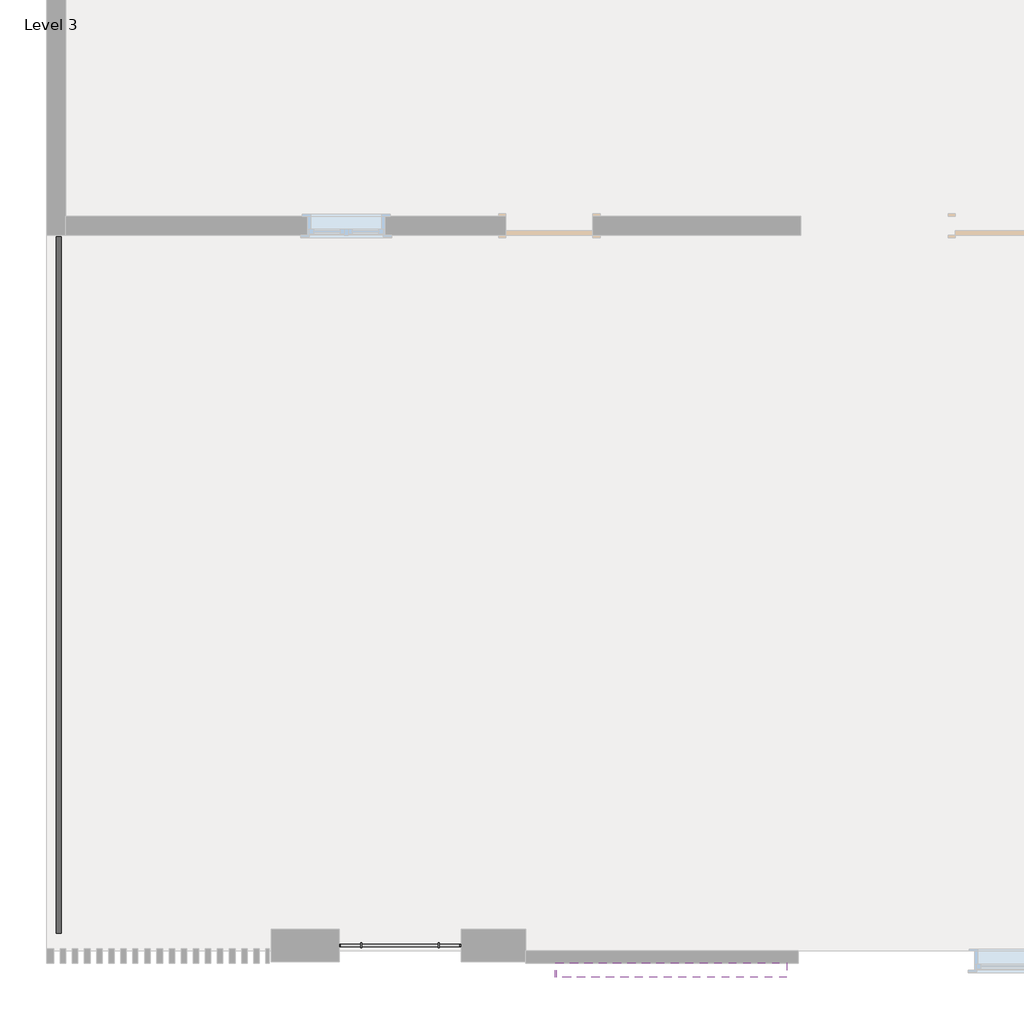
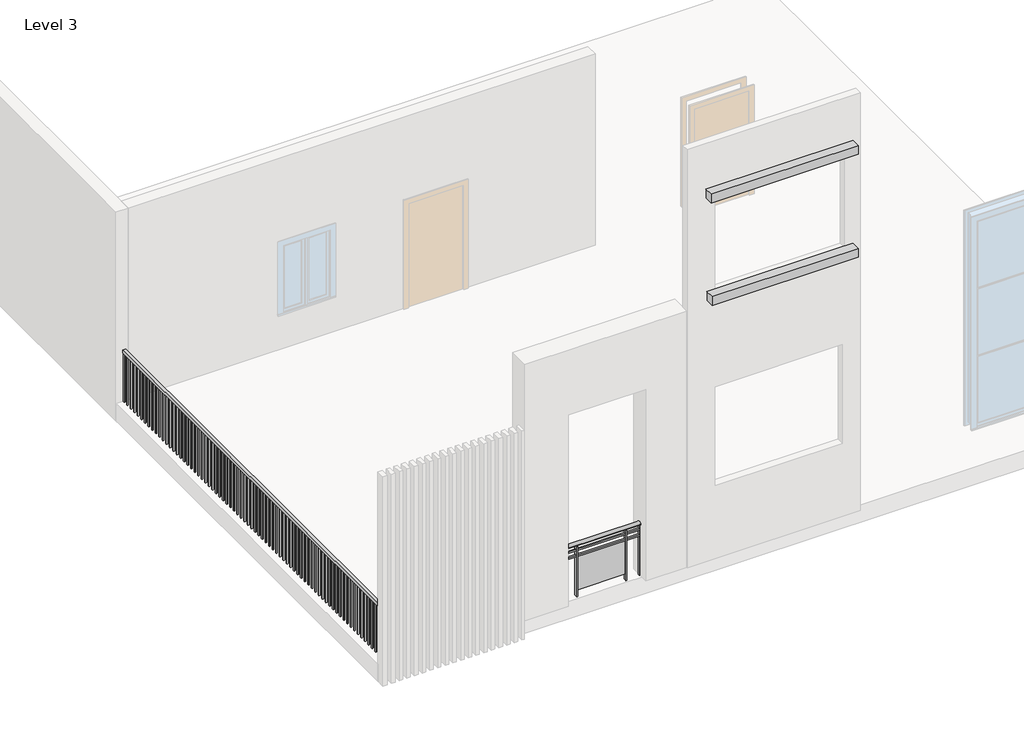
# One storey, part 2 of 2: 2 proxies, 2 railings.
"""IFC4 building model written with IfcOpenShell, lengths in millimetres."""

from ifc_helpers import new_model, si_unit, point, frame, origin, place, context, project, spatial, polyline, ellipse_curve, trimmed, outline, extrude, element, save
from ifc_brep_helpers import plane_surface, extruded_surface, advanced_brep

model = new_model("IFC4")

# Units and contexts
model_context = context("Model", 3, world=origin())
ifc_project = project(units=[si_unit("LENGTHUNIT", "METRE", prefix="MILLI")], contexts=[model_context])

# Site, building, storey
site = spatial("IfcSite", under=ifc_project)
building = spatial("IfcBuilding", under=site)
storey = spatial("IfcBuildingStorey", under=building, Name="Level 3", Elevation=7315.2)

# Proxies
placement = place(None, origin())
element("IfcBuildingElementProxy", 1, Name="Cornice", ObjectType="Cornice", at=placement, inside=storey, context=model_context, shape_type="SweptSolid", body=[
    extrude(outline(polyline([(-6506.8547188, -1061.9189974), (-6506.8547188, -909.5189974), (-4073.2084212, -909.5189974), (-4073.2084212, -1061.9189974), (-6506.8547188, -1061.9189974)])), frame((0.0, 0.0, 13989.7022407), z_axis=(0.0, 0.0, 1.0), x_axis=(1.0, 0.0, 0.0)), (0.0, 0.0, 1.0), 152.4),
])
element("IfcBuildingElementProxy", 2, Name="Cornice", ObjectType="Cornice", at=placement, inside=storey, context=model_context, shape_type="SweptSolid", body=[
    extrude(outline(polyline([(-6490.544029, -1061.9189974), (-6490.544029, -909.5189974), (-4073.2084212, -909.5189974), (-4073.2084212, -1061.9189974), (-6490.544029, -1061.9189974)])), frame((0.0, 0.0, 12192.0), z_axis=(0.0, 0.0, 1.0), x_axis=(1.0, 0.0, 0.0)), (0.0, 0.0, 1.0), 152.4),
])

# Railings
element("IfcRailing", 3, ObjectType="Glass Panel - Bottom Fill", at=placement, inside=storey, context=model_context, shape_type="SolidModel", body=[
    advanced_brep(
    [(-8777.0745124, -686.4386035, 8534.4), (-8777.0745124, -762.6386035, 8534.4), (-7495.2589248, -686.4386035, 8534.4), (-7495.2589248, -762.6386035, 8534.4)],
    [
        (0, 1, ellipse_curve(frame((-8777.0745124, -724.5386035, 8534.4), z_axis=(-1.0, 0.0, 0.0), x_axis=(0.0, -1.0, 0.0)), 38.1, 28.575)),
        (1, 0, ellipse_curve(frame((-8777.0745124, -724.5386035, 8534.4), z_axis=(-1.0, 0.0, 0.0), x_axis=(0.0, -1.0, 0.0)), 38.1, 28.575)),
        (2, 3, ellipse_curve(frame((-7495.2589248, -724.5386035, 8534.4), z_axis=(1.0, 0.0, 0.0), x_axis=(0.0, -1.0, 0.0)), 38.1, 28.575)),
        (3, 2, ellipse_curve(frame((-7495.2589248, -724.5386035, 8534.4), z_axis=(1.0, 0.0, 0.0), x_axis=(0.0, -1.0, 0.0)), 38.1, 28.575)),
        (0, 2),
        (3, 1),
    ],
    [
        plane_surface(frame((-8777.0745124, -724.5386035, 8534.4), z_axis=(-1.0, 0.0, 0.0), x_axis=(0.0, 1.0, 0.0))),
        plane_surface(frame((-7495.2589248, -724.5386035, 8534.4), z_axis=(1.0, 0.0, 0.0), x_axis=(0.0, 1.0, 0.0))),
        extruded_surface(trimmed(ellipse_curve(frame((-7495.2589248, -724.5386035, 8534.4), z_axis=(-1.0, 0.0, 0.0), x_axis=(0.0, -1.0, 0.0)), 38.1, 28.575), [point((-7495.2589248, -686.4386035, 8534.4))], [point((-7495.2589248, -762.6386035, 8534.4))], True, "CARTESIAN"), (-1281.8155876, 0.0, 0.0), 1281.8155876),
        extruded_surface(trimmed(ellipse_curve(frame((-7495.2589248, -724.5386035, 8534.4), z_axis=(-1.0, 0.0, 0.0), x_axis=(0.0, -1.0, 0.0)), 38.1, 28.575), [point((-7495.2589248, -762.6386035, 8534.4))], [point((-7495.2589248, -686.4386035, 8534.4))], True, "CARTESIAN"), (-1281.8155876, 0.0, 0.0), 1281.8155876),
    ],
    [
        (0, [[1, 2]]),
        (1, [[3, 4]]),
        (2, [[-1, 5, -4, 6]]),
        (3, [[-2, -6, -3, -5]]),
    ],
),
    extrude(outline(polyline([(-8777.0745124, -737.2386035), (-8777.0745124, -711.8386035), (-7495.2589248, -711.8386035), (-7495.2589248, -737.2386035), (-8777.0745124, -737.2386035)])), frame((0.0, 0.0, 8420.1), z_axis=(0.0, 0.0, 1.0), x_axis=(1.0, 0.0, 0.0)), (0.0, 0.0, 1.0), 25.4),
    extrude(outline(polyline([(-8777.0745124, -737.2386035), (-8777.0745124, -711.8386035), (-7495.2589248, -711.8386035), (-7495.2589248, -737.2386035), (-8777.0745124, -737.2386035)])), frame((0.0, 0.0, 8318.5), z_axis=(0.0, 0.0, 1.0), x_axis=(1.0, 0.0, 0.0)), (0.0, 0.0, 1.0), 25.4),
    extrude(outline(polyline([(-7736.1167186, -749.9386035), (-7736.1167186, -699.1386035), (-7723.4167186, -699.1386035), (-7723.4167186, -749.9386035), (-7736.1167186, -749.9386035)])), frame((0.0, 0.0, 7620.0), z_axis=(0.0, 0.0, 1.0), x_axis=(1.0, 0.0, 0.0)), (0.0, 0.0, 1.0), 885.6788223),
    extrude(outline(polyline([(-8542.5667186, -718.0034465), (-7729.7667186, -718.0034465), (-7729.7667186, -724.3534465), (-8542.5667186, -724.3534465), (-8542.5667186, -718.0034465)])), frame((0.0, 0.0, 7721.6), z_axis=(0.0, 0.0, 1.0), x_axis=(1.0, 0.0, 0.0)), (0.0, 0.0, 1.0), 596.9),
    extrude(outline(polyline([(-8548.9167186, -749.9386035), (-8548.9167186, -699.1386035), (-8536.2167186, -699.1386035), (-8536.2167186, -749.9386035), (-8548.9167186, -749.9386035)])), frame((0.0, 0.0, 7620.0), z_axis=(0.0, 0.0, 1.0), x_axis=(1.0, 0.0, 0.0)), (0.0, 0.0, 1.0), 885.6788223),
    extrude(outline(polyline([(-7507.9589248, -734.0636035), (-7507.9589248, -715.0136035), (-7488.9089248, -715.0136035), (-7488.9089248, -734.0636035), (-7507.9589248, -734.0636035)])), frame((0.0, 0.0, 7620.0), z_axis=(0.0, 0.0, 1.0), x_axis=(1.0, 0.0, 0.0)), (0.0, 0.0, 1.0), 885.6788223),
    extrude(outline(polyline([(-8783.4245124, -734.0636035), (-8783.4245124, -715.0136035), (-8764.3745124, -715.0136035), (-8764.3745124, -734.0636035), (-8783.4245124, -734.0636035)])), frame((0.0, 0.0, 7620.0), z_axis=(0.0, 0.0, 1.0), x_axis=(1.0, 0.0, 0.0)), (0.0, 0.0, 1.0), 885.6788223),
])
element("IfcRailing", 4, ObjectType="Handrail - Rectangular", at=placement, inside=storey, context=model_context, shape_type="SweptSolid", body=[
    extrude(outline(polyline([(-11748.8745124, 6720.6131791), (-11698.0745124, 6720.6131791), (-11698.0745124, -594.5868209), (-11748.8745124, -594.5868209), (-11748.8745124, 6720.6131791)])), frame((0.0, 0.0, 8483.6), z_axis=(0.0, 0.0, 1.0), x_axis=(1.0, 0.0, 0.0)), (0.0, 0.0, 1.0), 50.8),
    extrude(outline(polyline([(-11732.9995124, -483.4618209), (-11713.9495124, -483.4618209), (-11713.9495124, -502.5118209), (-11732.9995124, -502.5118209), (-11732.9995124, -483.4618209)])), frame((0.0, 0.0, 7620.0), z_axis=(0.0, 0.0, 1.0), x_axis=(1.0, 0.0, 0.0)), (0.0, 0.0, 1.0), 863.6),
    extrude(outline(polyline([(-11732.9995124, -381.8618209), (-11713.9495124, -381.8618209), (-11713.9495124, -400.9118209), (-11732.9995124, -400.9118209), (-11732.9995124, -381.8618209)])), frame((0.0, 0.0, 7620.0), z_axis=(0.0, 0.0, 1.0), x_axis=(1.0, 0.0, 0.0)), (0.0, 0.0, 1.0), 863.6),
    extrude(outline(polyline([(-11732.9995124, -280.2618209), (-11713.9495124, -280.2618209), (-11713.9495124, -299.3118209), (-11732.9995124, -299.3118209), (-11732.9995124, -280.2618209)])), frame((0.0, 0.0, 7620.0), z_axis=(0.0, 0.0, 1.0), x_axis=(1.0, 0.0, 0.0)), (0.0, 0.0, 1.0), 863.6),
    extrude(outline(polyline([(-11732.9995124, -178.6618209), (-11713.9495124, -178.6618209), (-11713.9495124, -197.7118209), (-11732.9995124, -197.7118209), (-11732.9995124, -178.6618209)])), frame((0.0, 0.0, 7620.0), z_axis=(0.0, 0.0, 1.0), x_axis=(1.0, 0.0, 0.0)), (0.0, 0.0, 1.0), 863.6),
    extrude(outline(polyline([(-11732.9995124, -77.0618209), (-11713.9495124, -77.0618209), (-11713.9495124, -96.1118209), (-11732.9995124, -96.1118209), (-11732.9995124, -77.0618209)])), frame((0.0, 0.0, 7620.0), z_axis=(0.0, 0.0, 1.0), x_axis=(1.0, 0.0, 0.0)), (0.0, 0.0, 1.0), 863.6),
    extrude(outline(polyline([(-11732.9995124, 24.5381791), (-11713.9495124, 24.5381791), (-11713.9495124, 5.4881791), (-11732.9995124, 5.4881791), (-11732.9995124, 24.5381791)])), frame((0.0, 0.0, 7620.0), z_axis=(0.0, 0.0, 1.0), x_axis=(1.0, 0.0, 0.0)), (0.0, 0.0, 1.0), 863.6),
    extrude(outline(polyline([(-11732.9995124, 126.1381791), (-11713.9495124, 126.1381791), (-11713.9495124, 107.0881791), (-11732.9995124, 107.0881791), (-11732.9995124, 126.1381791)])), frame((0.0, 0.0, 7620.0), z_axis=(0.0, 0.0, 1.0), x_axis=(1.0, 0.0, 0.0)), (0.0, 0.0, 1.0), 863.6),
    extrude(outline(polyline([(-11732.9995124, 227.7381791), (-11713.9495124, 227.7381791), (-11713.9495124, 208.6881791), (-11732.9995124, 208.6881791), (-11732.9995124, 227.7381791)])), frame((0.0, 0.0, 7620.0), z_axis=(0.0, 0.0, 1.0), x_axis=(1.0, 0.0, 0.0)), (0.0, 0.0, 1.0), 863.6),
    extrude(outline(polyline([(-11732.9995124, 329.3381791), (-11713.9495124, 329.3381791), (-11713.9495124, 310.2881791), (-11732.9995124, 310.2881791), (-11732.9995124, 329.3381791)])), frame((0.0, 0.0, 7620.0), z_axis=(0.0, 0.0, 1.0), x_axis=(1.0, 0.0, 0.0)), (0.0, 0.0, 1.0), 863.6),
    extrude(outline(polyline([(-11732.9995124, 430.9381791), (-11713.9495124, 430.9381791), (-11713.9495124, 411.8881791), (-11732.9995124, 411.8881791), (-11732.9995124, 430.9381791)])), frame((0.0, 0.0, 7620.0), z_axis=(0.0, 0.0, 1.0), x_axis=(1.0, 0.0, 0.0)), (0.0, 0.0, 1.0), 863.6),
    extrude(outline(polyline([(-11732.9995124, 532.5381791), (-11713.9495124, 532.5381791), (-11713.9495124, 513.4881791), (-11732.9995124, 513.4881791), (-11732.9995124, 532.5381791)])), frame((0.0, 0.0, 7620.0), z_axis=(0.0, 0.0, 1.0), x_axis=(1.0, 0.0, 0.0)), (0.0, 0.0, 1.0), 863.6),
    extrude(outline(polyline([(-11732.9995124, 634.1381791), (-11713.9495124, 634.1381791), (-11713.9495124, 615.0881791), (-11732.9995124, 615.0881791), (-11732.9995124, 634.1381791)])), frame((0.0, 0.0, 7620.0), z_axis=(0.0, 0.0, 1.0), x_axis=(1.0, 0.0, 0.0)), (0.0, 0.0, 1.0), 863.6),
    extrude(outline(polyline([(-11732.9995124, 735.7381791), (-11713.9495124, 735.7381791), (-11713.9495124, 716.6881791), (-11732.9995124, 716.6881791), (-11732.9995124, 735.7381791)])), frame((0.0, 0.0, 7620.0), z_axis=(0.0, 0.0, 1.0), x_axis=(1.0, 0.0, 0.0)), (0.0, 0.0, 1.0), 863.6),
    extrude(outline(polyline([(-11732.9995124, 837.3381791), (-11713.9495124, 837.3381791), (-11713.9495124, 818.2881791), (-11732.9995124, 818.2881791), (-11732.9995124, 837.3381791)])), frame((0.0, 0.0, 7620.0), z_axis=(0.0, 0.0, 1.0), x_axis=(1.0, 0.0, 0.0)), (0.0, 0.0, 1.0), 863.6),
    extrude(outline(polyline([(-11732.9995124, 938.9381791), (-11713.9495124, 938.9381791), (-11713.9495124, 919.8881791), (-11732.9995124, 919.8881791), (-11732.9995124, 938.9381791)])), frame((0.0, 0.0, 7620.0), z_axis=(0.0, 0.0, 1.0), x_axis=(1.0, 0.0, 0.0)), (0.0, 0.0, 1.0), 863.6),
    extrude(outline(polyline([(-11732.9995124, 1040.5381791), (-11713.9495124, 1040.5381791), (-11713.9495124, 1021.4881791), (-11732.9995124, 1021.4881791), (-11732.9995124, 1040.5381791)])), frame((0.0, 0.0, 7620.0), z_axis=(0.0, 0.0, 1.0), x_axis=(1.0, 0.0, 0.0)), (0.0, 0.0, 1.0), 863.6),
    extrude(outline(polyline([(-11732.9995124, 1142.1381791), (-11713.9495124, 1142.1381791), (-11713.9495124, 1123.0881791), (-11732.9995124, 1123.0881791), (-11732.9995124, 1142.1381791)])), frame((0.0, 0.0, 7620.0), z_axis=(0.0, 0.0, 1.0), x_axis=(1.0, 0.0, 0.0)), (0.0, 0.0, 1.0), 863.6),
    extrude(outline(polyline([(-11732.9995124, 1243.7381791), (-11713.9495124, 1243.7381791), (-11713.9495124, 1224.6881791), (-11732.9995124, 1224.6881791), (-11732.9995124, 1243.7381791)])), frame((0.0, 0.0, 7620.0), z_axis=(0.0, 0.0, 1.0), x_axis=(1.0, 0.0, 0.0)), (0.0, 0.0, 1.0), 863.6),
    extrude(outline(polyline([(-11732.9995124, 1345.3381791), (-11713.9495124, 1345.3381791), (-11713.9495124, 1326.2881791), (-11732.9995124, 1326.2881791), (-11732.9995124, 1345.3381791)])), frame((0.0, 0.0, 7620.0), z_axis=(0.0, 0.0, 1.0), x_axis=(1.0, 0.0, 0.0)), (0.0, 0.0, 1.0), 863.6),
    extrude(outline(polyline([(-11732.9995124, 1446.9381791), (-11713.9495124, 1446.9381791), (-11713.9495124, 1427.8881791), (-11732.9995124, 1427.8881791), (-11732.9995124, 1446.9381791)])), frame((0.0, 0.0, 7620.0), z_axis=(0.0, 0.0, 1.0), x_axis=(1.0, 0.0, 0.0)), (0.0, 0.0, 1.0), 863.6),
    extrude(outline(polyline([(-11732.9995124, 1548.5381791), (-11713.9495124, 1548.5381791), (-11713.9495124, 1529.4881791), (-11732.9995124, 1529.4881791), (-11732.9995124, 1548.5381791)])), frame((0.0, 0.0, 7620.0), z_axis=(0.0, 0.0, 1.0), x_axis=(1.0, 0.0, 0.0)), (0.0, 0.0, 1.0), 863.6),
    extrude(outline(polyline([(-11732.9995124, 1650.1381791), (-11713.9495124, 1650.1381791), (-11713.9495124, 1631.0881791), (-11732.9995124, 1631.0881791), (-11732.9995124, 1650.1381791)])), frame((0.0, 0.0, 7620.0), z_axis=(0.0, 0.0, 1.0), x_axis=(1.0, 0.0, 0.0)), (0.0, 0.0, 1.0), 863.6),
    extrude(outline(polyline([(-11732.9995124, 1751.7381791), (-11713.9495124, 1751.7381791), (-11713.9495124, 1732.6881791), (-11732.9995124, 1732.6881791), (-11732.9995124, 1751.7381791)])), frame((0.0, 0.0, 7620.0), z_axis=(0.0, 0.0, 1.0), x_axis=(1.0, 0.0, 0.0)), (0.0, 0.0, 1.0), 863.6),
    extrude(outline(polyline([(-11732.9995124, 1853.3381791), (-11713.9495124, 1853.3381791), (-11713.9495124, 1834.2881791), (-11732.9995124, 1834.2881791), (-11732.9995124, 1853.3381791)])), frame((0.0, 0.0, 7620.0), z_axis=(0.0, 0.0, 1.0), x_axis=(1.0, 0.0, 0.0)), (0.0, 0.0, 1.0), 863.6),
    extrude(outline(polyline([(-11732.9995124, 1954.9381791), (-11713.9495124, 1954.9381791), (-11713.9495124, 1935.8881791), (-11732.9995124, 1935.8881791), (-11732.9995124, 1954.9381791)])), frame((0.0, 0.0, 7620.0), z_axis=(0.0, 0.0, 1.0), x_axis=(1.0, 0.0, 0.0)), (0.0, 0.0, 1.0), 863.6),
    extrude(outline(polyline([(-11732.9995124, 2056.5381791), (-11713.9495124, 2056.5381791), (-11713.9495124, 2037.4881791), (-11732.9995124, 2037.4881791), (-11732.9995124, 2056.5381791)])), frame((0.0, 0.0, 7620.0), z_axis=(0.0, 0.0, 1.0), x_axis=(1.0, 0.0, 0.0)), (0.0, 0.0, 1.0), 863.6),
    extrude(outline(polyline([(-11732.9995124, 2158.1381791), (-11713.9495124, 2158.1381791), (-11713.9495124, 2139.0881791), (-11732.9995124, 2139.0881791), (-11732.9995124, 2158.1381791)])), frame((0.0, 0.0, 7620.0), z_axis=(0.0, 0.0, 1.0), x_axis=(1.0, 0.0, 0.0)), (0.0, 0.0, 1.0), 863.6),
    extrude(outline(polyline([(-11732.9995124, 2259.7381791), (-11713.9495124, 2259.7381791), (-11713.9495124, 2240.6881791), (-11732.9995124, 2240.6881791), (-11732.9995124, 2259.7381791)])), frame((0.0, 0.0, 7620.0), z_axis=(0.0, 0.0, 1.0), x_axis=(1.0, 0.0, 0.0)), (0.0, 0.0, 1.0), 863.6),
    extrude(outline(polyline([(-11732.9995124, 2361.3381791), (-11713.9495124, 2361.3381791), (-11713.9495124, 2342.2881791), (-11732.9995124, 2342.2881791), (-11732.9995124, 2361.3381791)])), frame((0.0, 0.0, 7620.0), z_axis=(0.0, 0.0, 1.0), x_axis=(1.0, 0.0, 0.0)), (0.0, 0.0, 1.0), 863.6),
    extrude(outline(polyline([(-11732.9995124, 2462.9381791), (-11713.9495124, 2462.9381791), (-11713.9495124, 2443.8881791), (-11732.9995124, 2443.8881791), (-11732.9995124, 2462.9381791)])), frame((0.0, 0.0, 7620.0), z_axis=(0.0, 0.0, 1.0), x_axis=(1.0, 0.0, 0.0)), (0.0, 0.0, 1.0), 863.6),
    extrude(outline(polyline([(-11732.9995124, 2564.5381791), (-11713.9495124, 2564.5381791), (-11713.9495124, 2545.4881791), (-11732.9995124, 2545.4881791), (-11732.9995124, 2564.5381791)])), frame((0.0, 0.0, 7620.0), z_axis=(0.0, 0.0, 1.0), x_axis=(1.0, 0.0, 0.0)), (0.0, 0.0, 1.0), 863.6),
    extrude(outline(polyline([(-11732.9995124, 2666.1381791), (-11713.9495124, 2666.1381791), (-11713.9495124, 2647.0881791), (-11732.9995124, 2647.0881791), (-11732.9995124, 2666.1381791)])), frame((0.0, 0.0, 7620.0), z_axis=(0.0, 0.0, 1.0), x_axis=(1.0, 0.0, 0.0)), (0.0, 0.0, 1.0), 863.6),
    extrude(outline(polyline([(-11732.9995124, 2767.7381791), (-11713.9495124, 2767.7381791), (-11713.9495124, 2748.6881791), (-11732.9995124, 2748.6881791), (-11732.9995124, 2767.7381791)])), frame((0.0, 0.0, 7620.0), z_axis=(0.0, 0.0, 1.0), x_axis=(1.0, 0.0, 0.0)), (0.0, 0.0, 1.0), 863.6),
    extrude(outline(polyline([(-11732.9995124, 2869.3381791), (-11713.9495124, 2869.3381791), (-11713.9495124, 2850.2881791), (-11732.9995124, 2850.2881791), (-11732.9995124, 2869.3381791)])), frame((0.0, 0.0, 7620.0), z_axis=(0.0, 0.0, 1.0), x_axis=(1.0, 0.0, 0.0)), (0.0, 0.0, 1.0), 863.6),
    extrude(outline(polyline([(-11732.9995124, 2970.9381791), (-11713.9495124, 2970.9381791), (-11713.9495124, 2951.8881791), (-11732.9995124, 2951.8881791), (-11732.9995124, 2970.9381791)])), frame((0.0, 0.0, 7620.0), z_axis=(0.0, 0.0, 1.0), x_axis=(1.0, 0.0, 0.0)), (0.0, 0.0, 1.0), 863.6),
    extrude(outline(polyline([(-11732.9995124, 3072.5381791), (-11713.9495124, 3072.5381791), (-11713.9495124, 3053.4881791), (-11732.9995124, 3053.4881791), (-11732.9995124, 3072.5381791)])), frame((0.0, 0.0, 7620.0), z_axis=(0.0, 0.0, 1.0), x_axis=(1.0, 0.0, 0.0)), (0.0, 0.0, 1.0), 863.6),
    extrude(outline(polyline([(-11732.9995124, 3174.1381791), (-11713.9495124, 3174.1381791), (-11713.9495124, 3155.0881791), (-11732.9995124, 3155.0881791), (-11732.9995124, 3174.1381791)])), frame((0.0, 0.0, 7620.0), z_axis=(0.0, 0.0, 1.0), x_axis=(1.0, 0.0, 0.0)), (0.0, 0.0, 1.0), 863.6),
    extrude(outline(polyline([(-11732.9995124, 3275.7381791), (-11713.9495124, 3275.7381791), (-11713.9495124, 3256.6881791), (-11732.9995124, 3256.6881791), (-11732.9995124, 3275.7381791)])), frame((0.0, 0.0, 7620.0), z_axis=(0.0, 0.0, 1.0), x_axis=(1.0, 0.0, 0.0)), (0.0, 0.0, 1.0), 863.6),
    extrude(outline(polyline([(-11732.9995124, 3377.3381791), (-11713.9495124, 3377.3381791), (-11713.9495124, 3358.2881791), (-11732.9995124, 3358.2881791), (-11732.9995124, 3377.3381791)])), frame((0.0, 0.0, 7620.0), z_axis=(0.0, 0.0, 1.0), x_axis=(1.0, 0.0, 0.0)), (0.0, 0.0, 1.0), 863.6),
    extrude(outline(polyline([(-11732.9995124, 3478.9381791), (-11713.9495124, 3478.9381791), (-11713.9495124, 3459.8881791), (-11732.9995124, 3459.8881791), (-11732.9995124, 3478.9381791)])), frame((0.0, 0.0, 7620.0), z_axis=(0.0, 0.0, 1.0), x_axis=(1.0, 0.0, 0.0)), (0.0, 0.0, 1.0), 863.6),
    extrude(outline(polyline([(-11732.9995124, 3580.5381791), (-11713.9495124, 3580.5381791), (-11713.9495124, 3561.4881791), (-11732.9995124, 3561.4881791), (-11732.9995124, 3580.5381791)])), frame((0.0, 0.0, 7620.0), z_axis=(0.0, 0.0, 1.0), x_axis=(1.0, 0.0, 0.0)), (0.0, 0.0, 1.0), 863.6),
    extrude(outline(polyline([(-11732.9995124, 3682.1381791), (-11713.9495124, 3682.1381791), (-11713.9495124, 3663.0881791), (-11732.9995124, 3663.0881791), (-11732.9995124, 3682.1381791)])), frame((0.0, 0.0, 7620.0), z_axis=(0.0, 0.0, 1.0), x_axis=(1.0, 0.0, 0.0)), (0.0, 0.0, 1.0), 863.6),
    extrude(outline(polyline([(-11732.9995124, 3783.7381791), (-11713.9495124, 3783.7381791), (-11713.9495124, 3764.6881791), (-11732.9995124, 3764.6881791), (-11732.9995124, 3783.7381791)])), frame((0.0, 0.0, 7620.0), z_axis=(0.0, 0.0, 1.0), x_axis=(1.0, 0.0, 0.0)), (0.0, 0.0, 1.0), 863.6),
    extrude(outline(polyline([(-11732.9995124, 3885.3381791), (-11713.9495124, 3885.3381791), (-11713.9495124, 3866.2881791), (-11732.9995124, 3866.2881791), (-11732.9995124, 3885.3381791)])), frame((0.0, 0.0, 7620.0), z_axis=(0.0, 0.0, 1.0), x_axis=(1.0, 0.0, 0.0)), (0.0, 0.0, 1.0), 863.6),
    extrude(outline(polyline([(-11732.9995124, 3986.9381791), (-11713.9495124, 3986.9381791), (-11713.9495124, 3967.8881791), (-11732.9995124, 3967.8881791), (-11732.9995124, 3986.9381791)])), frame((0.0, 0.0, 7620.0), z_axis=(0.0, 0.0, 1.0), x_axis=(1.0, 0.0, 0.0)), (0.0, 0.0, 1.0), 863.6),
    extrude(outline(polyline([(-11732.9995124, 4088.5381791), (-11713.9495124, 4088.5381791), (-11713.9495124, 4069.4881791), (-11732.9995124, 4069.4881791), (-11732.9995124, 4088.5381791)])), frame((0.0, 0.0, 7620.0), z_axis=(0.0, 0.0, 1.0), x_axis=(1.0, 0.0, 0.0)), (0.0, 0.0, 1.0), 863.6),
    extrude(outline(polyline([(-11732.9995124, 4190.1381791), (-11713.9495124, 4190.1381791), (-11713.9495124, 4171.0881791), (-11732.9995124, 4171.0881791), (-11732.9995124, 4190.1381791)])), frame((0.0, 0.0, 7620.0), z_axis=(0.0, 0.0, 1.0), x_axis=(1.0, 0.0, 0.0)), (0.0, 0.0, 1.0), 863.6),
    extrude(outline(polyline([(-11732.9995124, 4291.7381791), (-11713.9495124, 4291.7381791), (-11713.9495124, 4272.6881791), (-11732.9995124, 4272.6881791), (-11732.9995124, 4291.7381791)])), frame((0.0, 0.0, 7620.0), z_axis=(0.0, 0.0, 1.0), x_axis=(1.0, 0.0, 0.0)), (0.0, 0.0, 1.0), 863.6),
    extrude(outline(polyline([(-11732.9995124, 4393.3381791), (-11713.9495124, 4393.3381791), (-11713.9495124, 4374.2881791), (-11732.9995124, 4374.2881791), (-11732.9995124, 4393.3381791)])), frame((0.0, 0.0, 7620.0), z_axis=(0.0, 0.0, 1.0), x_axis=(1.0, 0.0, 0.0)), (0.0, 0.0, 1.0), 863.6),
    extrude(outline(polyline([(-11732.9995124, 4494.9381791), (-11713.9495124, 4494.9381791), (-11713.9495124, 4475.8881791), (-11732.9995124, 4475.8881791), (-11732.9995124, 4494.9381791)])), frame((0.0, 0.0, 7620.0), z_axis=(0.0, 0.0, 1.0), x_axis=(1.0, 0.0, 0.0)), (0.0, 0.0, 1.0), 863.6),
    extrude(outline(polyline([(-11732.9995124, 4596.5381791), (-11713.9495124, 4596.5381791), (-11713.9495124, 4577.4881791), (-11732.9995124, 4577.4881791), (-11732.9995124, 4596.5381791)])), frame((0.0, 0.0, 7620.0), z_axis=(0.0, 0.0, 1.0), x_axis=(1.0, 0.0, 0.0)), (0.0, 0.0, 1.0), 863.6),
    extrude(outline(polyline([(-11732.9995124, 4698.1381791), (-11713.9495124, 4698.1381791), (-11713.9495124, 4679.0881791), (-11732.9995124, 4679.0881791), (-11732.9995124, 4698.1381791)])), frame((0.0, 0.0, 7620.0), z_axis=(0.0, 0.0, 1.0), x_axis=(1.0, 0.0, 0.0)), (0.0, 0.0, 1.0), 863.6),
    extrude(outline(polyline([(-11732.9995124, 4799.7381791), (-11713.9495124, 4799.7381791), (-11713.9495124, 4780.6881791), (-11732.9995124, 4780.6881791), (-11732.9995124, 4799.7381791)])), frame((0.0, 0.0, 7620.0), z_axis=(0.0, 0.0, 1.0), x_axis=(1.0, 0.0, 0.0)), (0.0, 0.0, 1.0), 863.6),
    extrude(outline(polyline([(-11732.9995124, 4901.3381791), (-11713.9495124, 4901.3381791), (-11713.9495124, 4882.2881791), (-11732.9995124, 4882.2881791), (-11732.9995124, 4901.3381791)])), frame((0.0, 0.0, 7620.0), z_axis=(0.0, 0.0, 1.0), x_axis=(1.0, 0.0, 0.0)), (0.0, 0.0, 1.0), 863.6),
    extrude(outline(polyline([(-11732.9995124, 5002.9381791), (-11713.9495124, 5002.9381791), (-11713.9495124, 4983.8881791), (-11732.9995124, 4983.8881791), (-11732.9995124, 5002.9381791)])), frame((0.0, 0.0, 7620.0), z_axis=(0.0, 0.0, 1.0), x_axis=(1.0, 0.0, 0.0)), (0.0, 0.0, 1.0), 863.6),
    extrude(outline(polyline([(-11732.9995124, 5104.5381791), (-11713.9495124, 5104.5381791), (-11713.9495124, 5085.4881791), (-11732.9995124, 5085.4881791), (-11732.9995124, 5104.5381791)])), frame((0.0, 0.0, 7620.0), z_axis=(0.0, 0.0, 1.0), x_axis=(1.0, 0.0, 0.0)), (0.0, 0.0, 1.0), 863.6),
    extrude(outline(polyline([(-11732.9995124, 5206.1381791), (-11713.9495124, 5206.1381791), (-11713.9495124, 5187.0881791), (-11732.9995124, 5187.0881791), (-11732.9995124, 5206.1381791)])), frame((0.0, 0.0, 7620.0), z_axis=(0.0, 0.0, 1.0), x_axis=(1.0, 0.0, 0.0)), (0.0, 0.0, 1.0), 863.6),
    extrude(outline(polyline([(-11732.9995124, 5307.7381791), (-11713.9495124, 5307.7381791), (-11713.9495124, 5288.6881791), (-11732.9995124, 5288.6881791), (-11732.9995124, 5307.7381791)])), frame((0.0, 0.0, 7620.0), z_axis=(0.0, 0.0, 1.0), x_axis=(1.0, 0.0, 0.0)), (0.0, 0.0, 1.0), 863.6),
    extrude(outline(polyline([(-11732.9995124, 5409.3381791), (-11713.9495124, 5409.3381791), (-11713.9495124, 5390.2881791), (-11732.9995124, 5390.2881791), (-11732.9995124, 5409.3381791)])), frame((0.0, 0.0, 7620.0), z_axis=(0.0, 0.0, 1.0), x_axis=(1.0, 0.0, 0.0)), (0.0, 0.0, 1.0), 863.6),
    extrude(outline(polyline([(-11732.9995124, 5510.9381791), (-11713.9495124, 5510.9381791), (-11713.9495124, 5491.8881791), (-11732.9995124, 5491.8881791), (-11732.9995124, 5510.9381791)])), frame((0.0, 0.0, 7620.0), z_axis=(0.0, 0.0, 1.0), x_axis=(1.0, 0.0, 0.0)), (0.0, 0.0, 1.0), 863.6),
    extrude(outline(polyline([(-11732.9995124, 5612.5381791), (-11713.9495124, 5612.5381791), (-11713.9495124, 5593.4881791), (-11732.9995124, 5593.4881791), (-11732.9995124, 5612.5381791)])), frame((0.0, 0.0, 7620.0), z_axis=(0.0, 0.0, 1.0), x_axis=(1.0, 0.0, 0.0)), (0.0, 0.0, 1.0), 863.6),
    extrude(outline(polyline([(-11732.9995124, 5714.1381791), (-11713.9495124, 5714.1381791), (-11713.9495124, 5695.0881791), (-11732.9995124, 5695.0881791), (-11732.9995124, 5714.1381791)])), frame((0.0, 0.0, 7620.0), z_axis=(0.0, 0.0, 1.0), x_axis=(1.0, 0.0, 0.0)), (0.0, 0.0, 1.0), 863.6),
    extrude(outline(polyline([(-11732.9995124, 5815.7381791), (-11713.9495124, 5815.7381791), (-11713.9495124, 5796.6881791), (-11732.9995124, 5796.6881791), (-11732.9995124, 5815.7381791)])), frame((0.0, 0.0, 7620.0), z_axis=(0.0, 0.0, 1.0), x_axis=(1.0, 0.0, 0.0)), (0.0, 0.0, 1.0), 863.6),
    extrude(outline(polyline([(-11732.9995124, 5917.3381791), (-11713.9495124, 5917.3381791), (-11713.9495124, 5898.2881791), (-11732.9995124, 5898.2881791), (-11732.9995124, 5917.3381791)])), frame((0.0, 0.0, 7620.0), z_axis=(0.0, 0.0, 1.0), x_axis=(1.0, 0.0, 0.0)), (0.0, 0.0, 1.0), 863.6),
    extrude(outline(polyline([(-11732.9995124, 6018.9381791), (-11713.9495124, 6018.9381791), (-11713.9495124, 5999.8881791), (-11732.9995124, 5999.8881791), (-11732.9995124, 6018.9381791)])), frame((0.0, 0.0, 7620.0), z_axis=(0.0, 0.0, 1.0), x_axis=(1.0, 0.0, 0.0)), (0.0, 0.0, 1.0), 863.6),
    extrude(outline(polyline([(-11732.9995124, 6120.5381791), (-11713.9495124, 6120.5381791), (-11713.9495124, 6101.4881791), (-11732.9995124, 6101.4881791), (-11732.9995124, 6120.5381791)])), frame((0.0, 0.0, 7620.0), z_axis=(0.0, 0.0, 1.0), x_axis=(1.0, 0.0, 0.0)), (0.0, 0.0, 1.0), 863.6),
    extrude(outline(polyline([(-11732.9995124, 6222.1381791), (-11713.9495124, 6222.1381791), (-11713.9495124, 6203.0881791), (-11732.9995124, 6203.0881791), (-11732.9995124, 6222.1381791)])), frame((0.0, 0.0, 7620.0), z_axis=(0.0, 0.0, 1.0), x_axis=(1.0, 0.0, 0.0)), (0.0, 0.0, 1.0), 863.6),
    extrude(outline(polyline([(-11732.9995124, 6323.7381791), (-11713.9495124, 6323.7381791), (-11713.9495124, 6304.6881791), (-11732.9995124, 6304.6881791), (-11732.9995124, 6323.7381791)])), frame((0.0, 0.0, 7620.0), z_axis=(0.0, 0.0, 1.0), x_axis=(1.0, 0.0, 0.0)), (0.0, 0.0, 1.0), 863.6),
    extrude(outline(polyline([(-11732.9995124, 6425.3381791), (-11713.9495124, 6425.3381791), (-11713.9495124, 6406.2881791), (-11732.9995124, 6406.2881791), (-11732.9995124, 6425.3381791)])), frame((0.0, 0.0, 7620.0), z_axis=(0.0, 0.0, 1.0), x_axis=(1.0, 0.0, 0.0)), (0.0, 0.0, 1.0), 863.6),
    extrude(outline(polyline([(-11732.9995124, 6526.9381791), (-11713.9495124, 6526.9381791), (-11713.9495124, 6507.8881791), (-11732.9995124, 6507.8881791), (-11732.9995124, 6526.9381791)])), frame((0.0, 0.0, 7620.0), z_axis=(0.0, 0.0, 1.0), x_axis=(1.0, 0.0, 0.0)), (0.0, 0.0, 1.0), 863.6),
    extrude(outline(polyline([(-11732.9995124, 6628.5381791), (-11713.9495124, 6628.5381791), (-11713.9495124, 6609.4881791), (-11732.9995124, 6609.4881791), (-11732.9995124, 6628.5381791)])), frame((0.0, 0.0, 7620.0), z_axis=(0.0, 0.0, 1.0), x_axis=(1.0, 0.0, 0.0)), (0.0, 0.0, 1.0), 863.6),
    extrude(outline(polyline([(-11732.9995124, -575.5368209), (-11713.9495124, -575.5368209), (-11713.9495124, -594.5868209), (-11732.9995124, -594.5868209), (-11732.9995124, -575.5368209)])), frame((0.0, 0.0, 7620.0), z_axis=(0.0, 0.0, 1.0), x_axis=(1.0, 0.0, 0.0)), (0.0, 0.0, 1.0), 863.6),
    extrude(outline(polyline([(-11732.9995124, 6720.6131791), (-11713.9495124, 6720.6131791), (-11713.9495124, 6701.5631791), (-11732.9995124, 6701.5631791), (-11732.9995124, 6720.6131791)])), frame((0.0, 0.0, 7620.0), z_axis=(0.0, 0.0, 1.0), x_axis=(1.0, 0.0, 0.0)), (0.0, 0.0, 1.0), 863.6),
])

save(model, "model.ifc")

# Revit data of these elements
# Type "Glass Panel - Bottom Fill"
#   Assembly Code = "C2010400"
#   built-in parameter 1008612 = 0.0416667 (stored number, unit not read)
#   built-in parameter 1008611 = 0.0416667 (stored number, unit not read)
#   built-in parameter 1008609 = 0.333333 (stored number, unit not read)
#   built-in parameter 1008604 = 0.166667 (stored number, unit not read)
#   built-in parameter 1008603 = 0.166667 (stored number, unit not read)
#   Railing Height = 3' - 0"
#   built-in parameter 1008630 = 2
#   built-in parameter 1008610 = 2
#   built-in parameter 1008618 = Baluster - Square : 3/4"
# Type "Handrail - Rectangular"
#   Assembly Code = "C2010400"
#   built-in parameter 1008612 = 0.0416667 (stored number, unit not read)
#   built-in parameter 1008611 = 0.0416667 (stored number, unit not read)
#   built-in parameter 1008609 = 0.333333 (stored number, unit not read)
#   built-in parameter 1008604 = 0.166667 (stored number, unit not read)
#   built-in parameter 1008603 = 0.166667 (stored number, unit not read)
#   Railing Height = 3' - 0"
#   built-in parameter 1008630 = 2
#   built-in parameter 1008610 = 2
#   built-in parameter 1008618 = Baluster - Square : 3/4"
# Elements 1, 2 (IfcBuildingElementProxy, "Cornice")
#   Phase Created = New Construction
#   Materials on its faces: "Default Wall"
# Element 3 (IfcRailing, "Glass Panel - Bottom Fill")
#   built-in parameter 1008621 = 1 (stored number, unit not read)
#   Phase Created = New Construction
#   Materials on its faces: "Glass"
# Element 4 (IfcRailing, "Handrail - Rectangular")
#   built-in parameter 1008621 = 1 (stored number, unit not read)
#   Phase Created = New Construction
# Materials
#   "Default Wall": colour RGB 128 128 128, transparency 0
#   "Glass": class "Glass", colour RGB 0 128 192, transparency 0.75, Description = "Soda Lime Glass", Cost = 0
